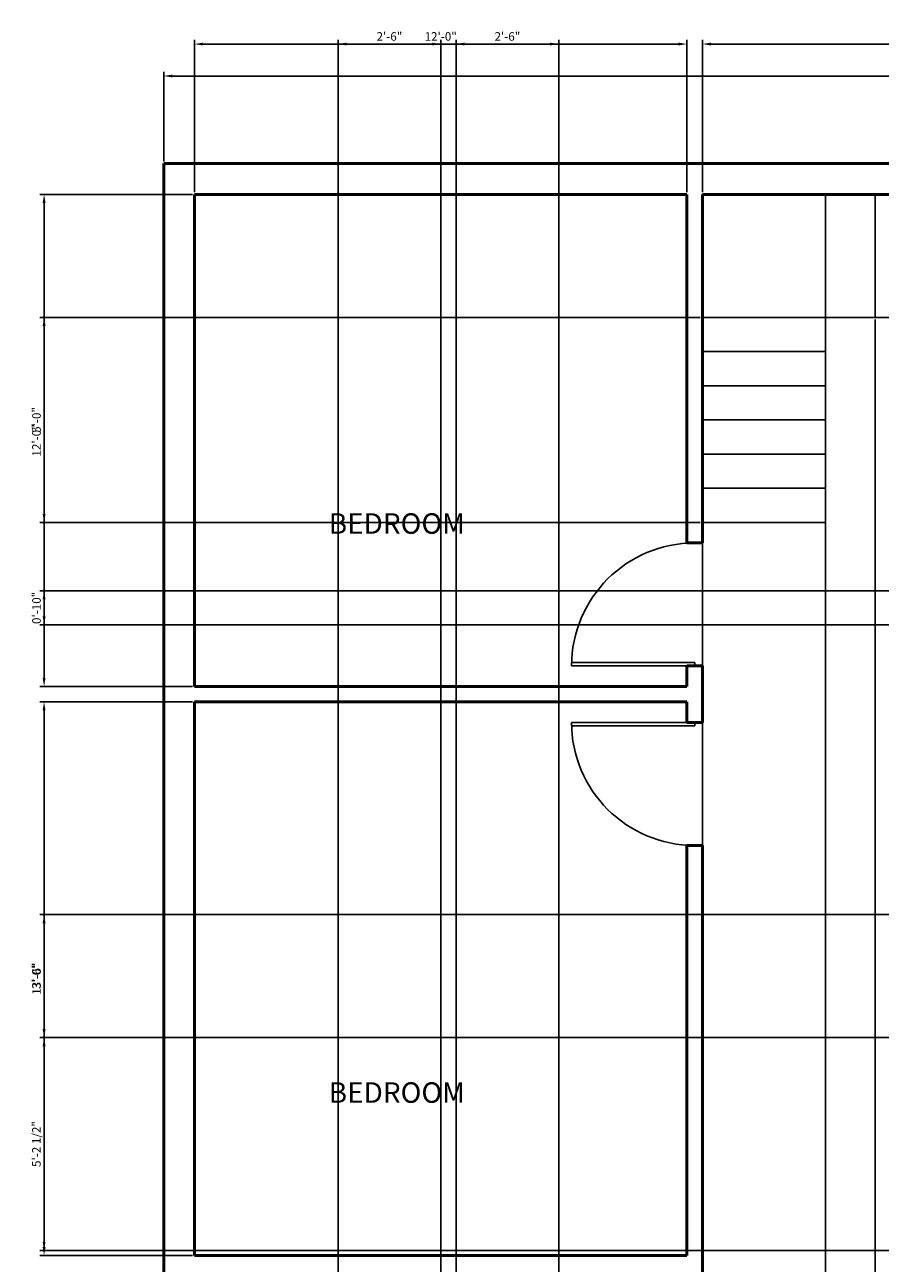
# Model space of a CAD drawing. Units: inches. Extents: x 877 to 2164, y 771 to 1603.
# Tile 2 of 6: x 1031 to 1281, y 1176 to 1538. Entities that reach past the tile are written whole.
import ezdxf

# ---------------------------------------------------------------- set-up
doc = ezdxf.new("R2010")
doc.units = ezdxf.units.IN
for name, color, linetype, lineweight in [('A-ANNO-DIMS', 2, 'Continuous', 18), ('A-AREA-IDEN', 7, 'Continuous', 25), ('A-DOOR', 5, 'Continuous', 25), ('A-FLOR-STRS', 7, 'Continuous', 25), ('A-WALL', 7, 'Continuous', 50)]:
    doc.layers.add(name, color=color, linetype=linetype, lineweight=lineweight)
doc.styles.get("Standard").update_dxf_attribs({"font": 'arial.ttf'})
doc.dimstyles.new('ISO-25', dxfattribs={"dimtxt": 2.5, "dimasz": 2.5, "dimexe": 1.25, "dimexo": 0.625, "dimtad": 1, "dimdec": 0, "dimlunit": 4, "dimtxsty": 'Standard', "dimcen": 2.5, "dimadec": 0, "dimazin": 0, "dimtfac": 1, "dimtdec": 0, "dimtmove": 0, "dimatfit": 3, "dimfxl": 1, "dimarcsym": 0})

# ---------------------------------------------------------------- blocks, each defined once
blk = doc.blocks.new('*D1')
at = {"layer": 'A-ANNO-DIMS', "color": 0, "lineweight": -2, "transparency": 16777216}
for p, q in [((1071.89, 1498.25), (1071.89, 1524.5)), ((1074.39, 1523.25), (1669.39, 1523.25)), ((1671.89, 1498.25), (1671.89, 1524.5))]:
    blk.add_line(p, q, dxfattribs=at)
at = {"layer": 'A-ANNO-DIMS', "color": 0, "transparency": 16777216}
for points in [[(1074.39, 1523.66), (1074.39, 1522.83), (1071.89, 1523.25)], [(1669.39, 1523.66), (1669.39, 1522.83), (1671.89, 1523.25)]]:
    blk.add_solid(points, dxfattribs=at)
at = {"layer": 'Defpoints', "color": 0, "transparency": 16777216}
for p in [(1671.89, 1523.25), (1071.89, 1497.62), (1671.89, 1497.62)]:
    blk.add_point(p, dxfattribs=at)
at = {"layer": 'A-ANNO-DIMS', "color": 0, "transparency": 16777216, "insert": (1371.89, 1525.15), "char_height": 2.5, "attachment_point": 5}
blk.add_mtext("50'", dxfattribs=at)
blk = doc.blocks.new('DOOR-SINGLE-36IN')
blk.add_lwpolyline([(0, 0), (0, 1), (36, 1), (36, 0)], close=True)
blk.add_arc((36, 0), 36, 90, 180)
blk = doc.blocks.new('*D10')
at = {"layer": 'A-ANNO-DIMS', "color": 0, "lineweight": -2, "transparency": 16777216}
for p, q in [((1080.89, 1489.25), (1080.89, 1533.85)), ((1224.89, 1489.25), (1224.89, 1533.85)), ((1083.39, 1532.6), (1222.39, 1532.6))]:
    blk.add_line(p, q, dxfattribs=at)
at = {"layer": 'A-ANNO-DIMS', "color": 0, "transparency": 16777216}
for points in [[(1083.39, 1533.01), (1083.39, 1532.18), (1080.89, 1532.6)], [(1222.39, 1533.01), (1222.39, 1532.18), (1224.89, 1532.6)]]:
    blk.add_solid(points, dxfattribs=at)
at = {"layer": 'Defpoints', "color": 0, "transparency": 16777216}
for p in [(1224.89, 1532.6), (1080.89, 1488.62), (1224.89, 1488.62)]:
    blk.add_point(p, dxfattribs=at)
at = {"layer": 'A-ANNO-DIMS', "color": 0, "transparency": 16777216, "insert": (1152.89, 1534.5), "char_height": 2.5, "attachment_point": 5}
blk.add_mtext('12\'-0"', dxfattribs=at)
blk = doc.blocks.new('*D11')
at = {"layer": 'A-ANNO-DIMS', "color": 0, "lineweight": -2, "transparency": 16777216}
for p, q in [((1229.39, 1489.25), (1229.39, 1533.85)), ((1365.89, 1489.25), (1365.89, 1533.85)), ((1231.89, 1532.6), (1363.39, 1532.6))]:
    blk.add_line(p, q, dxfattribs=at)
at = {"layer": 'A-ANNO-DIMS', "color": 0, "transparency": 16777216}
for points in [[(1231.89, 1533.01), (1231.89, 1532.18), (1229.39, 1532.6)], [(1363.39, 1533.01), (1363.39, 1532.18), (1365.89, 1532.6)]]:
    blk.add_solid(points, dxfattribs=at)
at = {"layer": 'Defpoints', "color": 0, "transparency": 16777216}
for p in [(1365.89, 1532.6), (1229.39, 1488.62), (1365.89, 1488.62)]:
    blk.add_point(p, dxfattribs=at)
at = {"layer": 'A-ANNO-DIMS', "color": 0, "transparency": 16777216, "insert": (1297.64, 1534.51), "char_height": 2.5, "attachment_point": 5}
blk.add_mtext('11\'-4 1/2"', dxfattribs=at)
blk = doc.blocks.new('*D14')
at = {"layer": 'A-ANNO-DIMS', "color": 0, "lineweight": -2, "transparency": 16777216}
for p, q in [((1080.27, 1488.62), (1035.67, 1488.62)), ((1036.92, 1347.12), (1036.92, 1486.12)), ((1080.27, 1344.62), (1035.67, 1344.62))]:
    blk.add_line(p, q, dxfattribs=at)
at = {"layer": 'A-ANNO-DIMS', "color": 0, "transparency": 16777216}
for points in [[(1036.5, 1486.12), (1037.34, 1486.12), (1036.92, 1488.62)], [(1036.5, 1347.12), (1037.34, 1347.12), (1036.92, 1344.62)]]:
    blk.add_solid(points, dxfattribs=at)
at = {"layer": 'Defpoints', "color": 0, "transparency": 16777216}
for p in [(1036.92, 1488.62), (1080.89, 1488.62), (1080.89, 1344.62)]:
    blk.add_point(p, dxfattribs=at)
at = {"layer": 'A-ANNO-DIMS', "color": 0, "transparency": 16777216, "insert": (1035.02, 1416.62), "char_height": 2.5, "attachment_point": 5, "rotation": 90}
blk.add_mtext('12\'-0"', dxfattribs=at)
blk = doc.blocks.new('*D15')
at = {"layer": 'A-ANNO-DIMS', "color": 0, "lineweight": -2, "transparency": 16777216}
for p, q in [((1080.27, 1340.12), (1035.67, 1340.12)), ((1036.92, 1180.62), (1036.92, 1337.62)), ((1080.27, 1178.12), (1035.67, 1178.12))]:
    blk.add_line(p, q, dxfattribs=at)
at = {"layer": 'A-ANNO-DIMS', "color": 0, "transparency": 16777216}
for points in [[(1036.5, 1337.62), (1037.34, 1337.62), (1036.92, 1340.12)], [(1036.5, 1180.62), (1037.34, 1180.62), (1036.92, 1178.12)]]:
    blk.add_solid(points, dxfattribs=at)
at = {"layer": 'Defpoints', "color": 0, "transparency": 16777216}
for p in [(1036.92, 1340.12), (1080.89, 1340.12), (1080.89, 1178.12)]:
    blk.add_point(p, dxfattribs=at)
at = {"layer": 'A-ANNO-DIMS', "color": 0, "transparency": 16777216, "insert": (1035.02, 1259.12), "char_height": 2.5, "attachment_point": 5, "rotation": 90}
blk.add_mtext('13\'-6"', dxfattribs=at)
blk = doc.blocks.new('*D19')
at = {"layer": 'A-ANNO-DIMS', "color": 0, "lineweight": -2, "transparency": 16777216}
for p, q in [((1567.77, 1277.87), (1035.67, 1277.87)), ((1036.92, 1244.37), (1036.92, 1275.37)), ((1567.77, 1241.87), (1035.67, 1241.87))]:
    blk.add_line(p, q, dxfattribs=at)
at = {"layer": 'A-ANNO-DIMS', "color": 0, "transparency": 16777216}
for points in [[(1036.5, 1275.37), (1037.34, 1275.37), (1036.92, 1277.87)], [(1036.5, 1244.37), (1037.34, 1244.37), (1036.92, 1241.87)]]:
    blk.add_solid(points, dxfattribs=at)
at = {"layer": 'Defpoints', "color": 0, "transparency": 16777216}
for p in [(1036.92, 1277.87), (1568.39, 1277.87), (1568.39, 1241.87)]:
    blk.add_point(p, dxfattribs=at)
at = {"layer": 'A-ANNO-DIMS', "color": 0, "transparency": 16777216, "insert": (1035.02, 1259.87), "char_height": 2.5, "attachment_point": 5, "rotation": 90}
blk.add_mtext('3\'-0"', dxfattribs=at)
blk = doc.blocks.new('*D20')
at = {"layer": 'A-ANNO-DIMS', "color": 0, "lineweight": -2, "transparency": 16777216}
for p, q in [((1567.77, 1241.87), (1035.67, 1241.87)), ((1036.92, 1182.12), (1036.92, 1239.37)), ((1572.27, 1179.62), (1035.67, 1179.62))]:
    blk.add_line(p, q, dxfattribs=at)
at = {"layer": 'A-ANNO-DIMS', "color": 0, "transparency": 16777216}
for points in [[(1036.5, 1239.37), (1037.34, 1239.37), (1036.92, 1241.87)], [(1036.5, 1182.12), (1037.34, 1182.12), (1036.92, 1179.62)]]:
    blk.add_solid(points, dxfattribs=at)
at = {"layer": 'Defpoints', "color": 0, "transparency": 16777216}
for p in [(1036.92, 1241.87), (1568.39, 1241.87), (1572.89, 1179.62)]:
    blk.add_point(p, dxfattribs=at)
at = {"layer": 'A-ANNO-DIMS', "color": 0, "transparency": 16777216, "insert": (1035, 1210.75), "char_height": 2.5, "attachment_point": 5, "rotation": 90}
blk.add_mtext('5\'-2 1/2"', dxfattribs=at)
blk = doc.blocks.new('*D34')
at = {"layer": 'A-ANNO-DIMS', "color": 0, "lineweight": -2, "transparency": 16777216}
for p, q in [((1122.89, 947.75), (1122.89, 1533.85)), ((1152.89, 947.75), (1152.89, 1533.85)), ((1125.39, 1532.6), (1150.39, 1532.6))]:
    blk.add_line(p, q, dxfattribs=at)
at = {"layer": 'A-ANNO-DIMS', "color": 0, "transparency": 16777216}
for points in [[(1125.39, 1533.01), (1125.39, 1532.18), (1122.89, 1532.6)], [(1150.39, 1533.01), (1150.39, 1532.18), (1152.89, 1532.6)]]:
    blk.add_solid(points, dxfattribs=at)
at = {"layer": 'Defpoints', "color": 0, "transparency": 16777216}
for p in [(1152.89, 1532.6), (1122.89, 947.12), (1152.89, 947.12)]:
    blk.add_point(p, dxfattribs=at)
at = {"layer": 'A-ANNO-DIMS', "color": 0, "transparency": 16777216, "insert": (1137.89, 1534.5), "char_height": 2.5, "attachment_point": 5}
blk.add_mtext('2\'-6"', dxfattribs=at)
blk = doc.blocks.new('*D35')
at = {"layer": 'A-ANNO-DIMS', "color": 0, "lineweight": -2, "transparency": 16777216}
for p, q in [((1157.39, 947.75), (1157.39, 1533.85)), ((1187.39, 947.75), (1187.39, 1533.85)), ((1159.89, 1532.6), (1184.89, 1532.6))]:
    blk.add_line(p, q, dxfattribs=at)
at = {"layer": 'A-ANNO-DIMS', "color": 0, "transparency": 16777216}
for points in [[(1159.89, 1533.01), (1159.89, 1532.18), (1157.39, 1532.6)], [(1184.89, 1533.01), (1184.89, 1532.18), (1187.39, 1532.6)]]:
    blk.add_solid(points, dxfattribs=at)
at = {"layer": 'Defpoints', "color": 0, "transparency": 16777216}
for p in [(1187.39, 1532.6), (1157.39, 947.12), (1187.39, 947.12)]:
    blk.add_point(p, dxfattribs=at)
at = {"layer": 'A-ANNO-DIMS', "color": 0, "transparency": 16777216, "insert": (1172.39, 1534.5), "char_height": 2.5, "attachment_point": 5}
blk.add_mtext('2\'-6"', dxfattribs=at)
blk = doc.blocks.new('*D37')
at = {"layer": 'A-ANNO-DIMS', "color": 0, "lineweight": -2, "transparency": 16777216}
for p, q in [((1229.39, 1392), (1229.39, 771.4)), ((1265.39, 1392), (1265.39, 771.4)), ((1231.89, 772.65), (1262.89, 772.65))]:
    blk.add_line(p, q, dxfattribs=at)
at = {"layer": 'A-ANNO-DIMS', "color": 0, "transparency": 16777216}
for points in [[(1231.89, 773.06), (1231.89, 772.23), (1229.39, 772.65)], [(1262.89, 773.06), (1262.89, 772.23), (1265.39, 772.65)]]:
    blk.add_solid(points, dxfattribs=at)
at = {"layer": 'Defpoints', "color": 0, "transparency": 16777216}
for p in [(1229.39, 1392.62), (1265.39, 1392.62), (1265.39, 772.65)]:
    blk.add_point(p, dxfattribs=at)
at = {"layer": 'A-ANNO-DIMS', "color": 0, "transparency": 16777216, "insert": (1247.39, 774.55), "char_height": 2.5, "attachment_point": 5}
blk.add_mtext('3\'-0"', dxfattribs=at)
blk = doc.blocks.new('*D40')
at = {"layer": 'A-ANNO-DIMS', "color": 0, "lineweight": -2, "transparency": 16777216}
for p, q in [((1228.77, 1452.62), (1035.67, 1452.62)), ((1036.92, 1395.12), (1036.92, 1450.12)), ((1228.77, 1392.62), (1035.67, 1392.62))]:
    blk.add_line(p, q, dxfattribs=at)
at = {"layer": 'A-ANNO-DIMS', "color": 0, "transparency": 16777216}
for points in [[(1036.5, 1450.12), (1037.34, 1450.12), (1036.92, 1452.62)], [(1036.5, 1395.12), (1037.34, 1395.12), (1036.92, 1392.62)]]:
    blk.add_solid(points, dxfattribs=at)
at = {"layer": 'Defpoints', "color": 0, "transparency": 16777216}
for p in [(1036.92, 1452.62), (1229.39, 1452.62), (1229.39, 1392.62)]:
    blk.add_point(p, dxfattribs=at)
at = {"layer": 'A-ANNO-DIMS', "color": 0, "transparency": 16777216, "insert": (1035.02, 1422.62), "char_height": 2.5, "attachment_point": 5, "rotation": 90}
blk.add_mtext('5\'-0"', dxfattribs=at)
blk = doc.blocks.new('*D41')
at = {"layer": 'A-ANNO-DIMS', "color": 0, "lineweight": -2, "transparency": 16777216}
for p, q in [((1329.27, 1372.62), (1035.67, 1372.62)), ((1036.92, 1365.12), (1036.92, 1370.12)), ((1329.27, 1362.62), (1035.67, 1362.62))]:
    blk.add_line(p, q, dxfattribs=at)
at = {"layer": 'A-ANNO-DIMS', "color": 0, "transparency": 16777216}
for points in [[(1036.5, 1370.12), (1037.34, 1370.12), (1036.92, 1372.62)], [(1036.5, 1365.12), (1037.34, 1365.12), (1036.92, 1362.62)]]:
    blk.add_solid(points, dxfattribs=at)
at = {"layer": 'Defpoints', "color": 0, "transparency": 16777216}
for p in [(1036.92, 1372.62), (1329.89, 1372.62), (1329.89, 1362.62)]:
    blk.add_point(p, dxfattribs=at)
at = {"layer": 'A-ANNO-DIMS', "color": 0, "transparency": 16777216, "insert": (1035.02, 1367.62), "char_height": 2.5, "attachment_point": 5, "rotation": 90}
blk.add_mtext('0\'-10"', dxfattribs=at)
blk = doc.blocks.new('*D43')
at = {"layer": 'A-ANNO-DIMS', "color": 0, "lineweight": -2, "transparency": 16777216}
for p, q in [((1279.89, 1452), (1279.89, 771.4)), ((1265.39, 1442), (1265.39, 771.4)), ((1267.89, 772.65), (1277.39, 772.65))]:
    blk.add_line(p, q, dxfattribs=at)
at = {"layer": 'A-ANNO-DIMS', "color": 0, "transparency": 16777216}
for points in [[(1267.89, 773.06), (1267.89, 772.23), (1265.39, 772.65)], [(1277.39, 773.06), (1277.39, 772.23), (1279.89, 772.65)]]:
    blk.add_solid(points, dxfattribs=at)
at = {"layer": 'Defpoints', "color": 0, "transparency": 16777216}
for p in [(1279.89, 1452.62), (1265.39, 1442.62), (1279.89, 772.65)]:
    blk.add_point(p, dxfattribs=at)
at = {"layer": 'A-ANNO-DIMS', "color": 0, "transparency": 16777216, "insert": (1272.64, 774.56), "char_height": 2.5, "attachment_point": 5}
blk.add_mtext('1\'-2 1/2"', dxfattribs=at)
blk = doc.blocks.new('*D44')
at = {"layer": 'A-ANNO-DIMS', "color": 0, "lineweight": -2, "transparency": 16777216}
for p, q in [((1279.89, 1452), (1279.89, 771.4)), ((1289.89, 1452), (1289.89, 771.4)), ((1282.39, 772.65), (1287.39, 772.65))]:
    blk.add_line(p, q, dxfattribs=at)
at = {"layer": 'A-ANNO-DIMS', "color": 0, "transparency": 16777216}
for points in [[(1282.39, 773.06), (1282.39, 772.23), (1279.89, 772.65)], [(1287.39, 773.06), (1287.39, 772.23), (1289.89, 772.65)]]:
    blk.add_solid(points, dxfattribs=at)
at = {"layer": 'Defpoints', "color": 0, "transparency": 16777216}
for p in [(1279.89, 1452.62), (1289.89, 1452.62), (1289.89, 772.65)]:
    blk.add_point(p, dxfattribs=at)
at = {"layer": 'A-ANNO-DIMS', "color": 0, "transparency": 16777216, "insert": (1284.89, 774.55), "char_height": 2.5, "attachment_point": 5}
blk.add_mtext('0\'-10"', dxfattribs=at)

msp = doc.modelspace()

# ---------------------------------------------------------------- linework, layer by layer
at = {"layer": 'A-FLOR-STRS'}
for p, q in [((1265.39, 1392.62), (1265.39, 1488.62)), ((1279.89, 1488.62), (1279.89, 1452.62)), ((1229.39, 1452.62), (1365.89, 1452.62)), ((1229.39, 1442.62), (1265.39, 1442.62)), ((1229.39, 1432.62), (1265.39, 1432.62)), ((1229.39, 1422.62), (1265.39, 1422.62)), ((1229.39, 1412.62), (1265.39, 1412.62)), ((1229.39, 1402.62), (1265.39, 1402.62)), ((1229.39, 1392.62), (1265.39, 1392.62))]:
    msp.add_line(p, q, dxfattribs=at)
at = {"layer": 'A-WALL'}
for p, q in [((1071.89, 837.62), (1071.89, 1497.62)), ((1071.89, 1497.62), (1671.89, 1497.62)), ((1080.89, 1488.62), (1224.89, 1488.62)), ((1080.89, 1344.62), (1080.89, 1488.62)), ((1224.89, 1386.62), (1224.89, 1488.62)), ((1229.39, 1386.62), (1229.39, 1488.62)), ((1229.39, 1488.62), (1365.89, 1488.62)), ((1224.89, 1386.62), (1229.39, 1386.62)), ((1224.89, 1344.62), (1224.89, 1350.62)), ((1224.89, 1350.62), (1229.39, 1350.62)), ((1229.39, 1334.12), (1229.39, 1350.62)), ((1080.89, 1344.62), (1224.89, 1344.62)), ((1080.89, 1340.12), (1224.89, 1340.12)), ((1080.89, 1178.12), (1080.89, 1340.12)), ((1224.89, 1334.12), (1224.89, 1340.12)), ((1224.89, 1334.12), (1229.39, 1334.12)), ((1224.89, 1298.12), (1229.39, 1298.12)), ((1224.89, 1178.12), (1224.89, 1298.12)), ((1229.39, 1167.62), (1229.39, 1298.12)), ((1080.89, 1178.12), (1224.89, 1178.12))]:
    msp.add_line(p, q, dxfattribs=at)

# ---------------------------------------------------------------- block references
at = {"layer": 'A-DOOR'}
msp.add_blockref('DOOR-SINGLE-36IN', (1191.15, 1350.62), dxfattribs=at)
at = {"layer": 'A-DOOR', "extrusion": (0, 0, -1), "zscale": -1, "rotation": 180}
msp.add_blockref('DOOR-SINGLE-36IN', (-1191.15, 1334.12), dxfattribs=at)

# ---------------------------------------------------------------- texts
at = {"layer": 'A-AREA-IDEN', "char_height": 6, "attachment_point": 1}
for insert in [(1120.14, 1395.31), (1120.14, 1228.81)]:
    msp.add_mtext_dynamic_manual_height_columns('BEDROOM', width=54.8109, gutter_width=12.5, heights=[0], dxfattribs=dict(at, insert=insert))

# ---------------------------------------------------------------- dimensions: what is measured, and where the dimension line sits
at = {"layer": 'A-ANNO-DIMS'}
for base, p1, p2, override, picture, middle in [((1365.89, 1532.6), (1229.39, 1488.62), (1365.89, 1488.62), {"dimdec": 1, "dimlfac": 1, "dimrnd": 0, "dimzin": 1, "dimdsep": 46, "dimlunit": 4, "dimfrac": 2}, '*D11', (1297.64, 1534.51)), ((1224.89, 1532.6), (1080.89, 1488.62), (1224.89, 1488.62), {"dimdec": 1, "dimlfac": 1, "dimrnd": 0, "dimzin": 1, "dimdsep": 46, "dimlunit": 4, "dimfrac": 2}, '*D10', (1152.89, 1534.5)), ((1152.89, 1532.6), (1122.89, 947.12), (1152.89, 947.12), {"dimdec": 1, "dimlfac": 1, "dimrnd": 0, "dimzin": 1, "dimdsep": 46, "dimlunit": 4, "dimfrac": 2}, '*D34', (1137.89, 1534.5)), ((1187.39, 1532.6), (1157.39, 947.12), (1187.39, 947.12), {"dimdec": 1, "dimlfac": 1, "dimrnd": 0, "dimzin": 1, "dimdsep": 46, "dimlunit": 4, "dimfrac": 2}, '*D35', (1172.39, 1534.5)), ((1671.89, 1523.25), (1071.89, 1497.62), (1671.89, 1497.62), {"dimclrd": 0, "dimclre": 0, "dimclrt": 0}, '*D1', (1371.89, 1525.15)), ((1279.89, 772.65), (1265.39, 1442.62), (1279.89, 1452.62), {"dimdec": 1, "dimlfac": 1, "dimrnd": 0, "dimzin": 1, "dimdsep": 46, "dimlunit": 4, "dimfrac": 2}, '*D43', (1272.64, 774.56)), ((1289.89, 772.65), (1279.89, 1452.62), (1289.89, 1452.62), {"dimdec": 1, "dimlfac": 1, "dimrnd": 0, "dimzin": 1, "dimdsep": 46, "dimlunit": 4, "dimfrac": 2}, '*D44', (1284.89, 774.55)), ((1265.39, 772.65), (1229.39, 1392.62), (1265.39, 1392.62), {"dimdec": 1, "dimlfac": 1, "dimrnd": 0, "dimzin": 1, "dimdsep": 46, "dimlunit": 4, "dimfrac": 2}, '*D37', (1247.39, 774.55))]:
    dim = msp.add_linear_dim(base=base, p1=p1, p2=p2, dimstyle='ISO-25', override=override, dxfattribs=at)
    dim.commit()
    dim.dimension.update_dxf_attribs({"geometry": picture, "text_midpoint": middle})
for base, p1, p2, picture, middle in [((1036.92, 1488.62), (1080.89, 1344.62), (1080.89, 1488.62), '*D14', (1035.02, 1416.62)), ((1036.92, 1452.62), (1229.39, 1392.62), (1229.39, 1452.62), '*D40', (1035.02, 1422.62)), ((1036.92, 1372.62), (1329.89, 1362.62), (1329.89, 1372.62), '*D41', (1035.02, 1367.62)), ((1036.92, 1340.12), (1080.89, 1178.12), (1080.89, 1340.12), '*D15', (1035.02, 1259.12)), ((1036.92, 1277.87), (1568.39, 1241.87), (1568.39, 1277.87), '*D19', (1035.02, 1259.87)), ((1036.91999, 1241.870352), (1572.89499, 1179.620352), (1568.39499, 1241.870352), '*D20', (1035.00235698, 1210.745352))]:
    dim = msp.add_linear_dim(base=base, p1=p1, p2=p2, angle=90, dimstyle='ISO-25', override={"dimdec": 1, "dimlfac": 1, "dimrnd": 0, "dimzin": 1, "dimdsep": 46, "dimlunit": 4, "dimfrac": 2}, dxfattribs=at)
    dim.commit()
    dim.dimension.update_dxf_attribs({"geometry": picture, "text_midpoint": middle})

doc.saveas('drawing.dxf')
